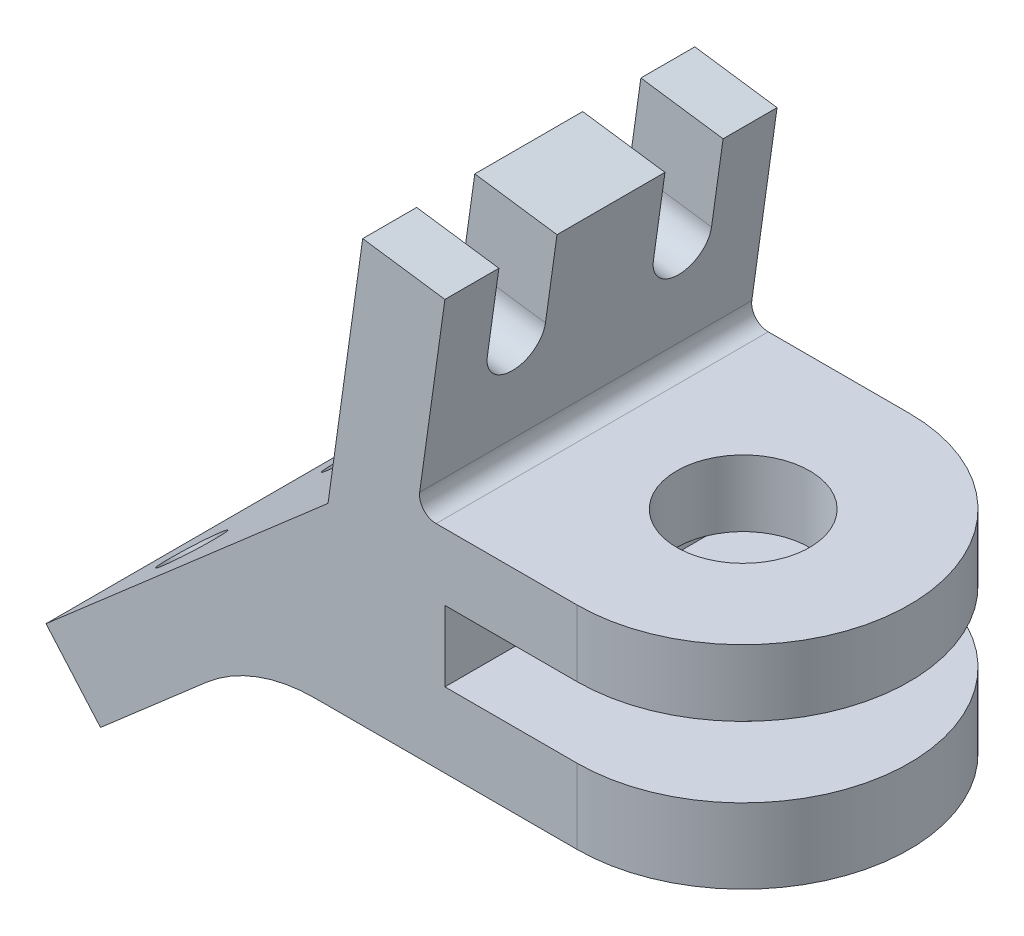
ISO-10303-21;
HEADER;
FILE_DESCRIPTION(('STEP AP214'),'2;1');
FILE_NAME('part.step','',(''),(''),'','','');
FILE_SCHEMA(('AUTOMOTIVE_DESIGN { 1 0 10303 214 1 1 1 1 }'));
ENDSEC;
DATA;
#1=APPLICATION_CONTEXT('core data for automotive mechanical design processes');
#2=APPLICATION_PROTOCOL_DEFINITION('international standard','automotive_design',2000,#1);
#3=PRODUCT_CONTEXT('',#1,'mechanical');
#4=PRODUCT('Part','Part','',(#3));
#5=PRODUCT_RELATED_PRODUCT_CATEGORY('part','',(#4));
#6=PRODUCT_DEFINITION_FORMATION('','',#4);
#7=PRODUCT_DEFINITION_CONTEXT('part definition',#1,'design');
#8=PRODUCT_DEFINITION('design','',#6,#7);
#9=PRODUCT_DEFINITION_SHAPE('','',#8);
#10=(LENGTH_UNIT() NAMED_UNIT(*) SI_UNIT(.MILLI.,.METRE.));
#11=(NAMED_UNIT(*) PLANE_ANGLE_UNIT() SI_UNIT($,.RADIAN.));
#12=(NAMED_UNIT(*) SI_UNIT($,.STERADIAN.) SOLID_ANGLE_UNIT());
#13=UNCERTAINTY_MEASURE_WITH_UNIT(LENGTH_MEASURE(1.E-05),#10,'distance_accuracy_value','');
#14=(GEOMETRIC_REPRESENTATION_CONTEXT(3) GLOBAL_UNCERTAINTY_ASSIGNED_CONTEXT((#13)) GLOBAL_UNIT_ASSIGNED_CONTEXT((#10,
#11,#12)) REPRESENTATION_CONTEXT('',''));
#15=CARTESIAN_POINT('',(0.,0.,0.));
#16=DIRECTION('',(0.,0.,1.));
#17=DIRECTION('',(1.,0.,0.));
#18=AXIS2_PLACEMENT_3D('',#15,#16,#17);
#19=CARTESIAN_POINT('',(0.,0.,4.));
#20=DIRECTION('',(-0.656059028990504,0.754709580222775,0.));
#21=DIRECTION('',(-0.754709580222775,-0.656059028990504,0.));
#22=AXIS2_PLACEMENT_3D('',#19,#20,#21);
#23=PLANE('',#22);
#24=CARTESIAN_POINT('',(-5.84731576057085,-5.08299404248799,-2.));
#25=DIRECTION('',(-0.656059028990504,0.754709580222775,0.));
#26=DIRECTION('',(-0.754709580222775,-0.656059028990504,0.));
#27=AXIS2_PLACEMENT_3D('',#24,#25,#26);
#28=CIRCLE('',#27,0.7);
#29=CARTESIAN_POINT('',(-6.37561246672679,-5.54223536278135,-2.));
#30=VERTEX_POINT('',#29);
#31=EDGE_CURVE('E244',#30,#30,#28,.T.);
#32=ORIENTED_EDGE('',*,*,#31,.T.);
#33=EDGE_LOOP('',(#32));
#34=FACE_BOUND('',#33,.T.);
#35=CARTESIAN_POINT('',(-5.84731576057085,-5.08299404248799,2.));
#36=DIRECTION('',(-0.656059028990504,0.754709580222775,0.));
#37=DIRECTION('',(-0.754709580222775,-0.656059028990504,0.));
#38=AXIS2_PLACEMENT_3D('',#35,#36,#37);
#39=CIRCLE('',#38,0.7);
#40=CARTESIAN_POINT('',(-6.37561246672679,-5.54223536278134,2.));
#41=VERTEX_POINT('',#40);
#42=EDGE_CURVE('E248',#41,#41,#39,.T.);
#43=ORIENTED_EDGE('',*,*,#42,.T.);
#44=EDGE_LOOP('',(#43));
#45=FACE_BOUND('',#44,.T.);
#46=DIRECTION('',(0.754709580222775,0.656059028990504,0.));
#47=VECTOR('',#46,1.);
#48=CARTESIAN_POINT('',(0.,0.,-4.));
#49=LINE('',#48,#47);
#50=CARTESIAN_POINT('',(-7.3567349210164,-6.395112100469,-4.));
#51=VERTEX_POINT('',#50);
#52=CARTESIAN_POINT('',(-4.80987630113007,-4.1811616791089,-4.));
#53=VERTEX_POINT('',#52);
#54=EDGE_CURVE('E325',#51,#53,#49,.T.);
#55=ORIENTED_EDGE('',*,*,#54,.T.);
#56=DIRECTION('',(0.,0.,-1.));
#57=VECTOR('',#56,1.);
#58=CARTESIAN_POINT('',(-4.80987630113007,-4.1811616791089,4.));
#59=LINE('',#58,#57);
#60=CARTESIAN_POINT('',(-4.80987630113007,-4.1811616791089,4.));
#61=VERTEX_POINT('',#60);
#62=EDGE_CURVE('E354',#53,#61,#59,.F.);
#63=ORIENTED_EDGE('',*,*,#62,.T.);
#64=DIRECTION('',(0.754709580222775,0.656059028990504,0.));
#65=VECTOR('',#64,1.);
#66=CARTESIAN_POINT('',(0.,0.,4.));
#67=LINE('',#66,#65);
#68=CARTESIAN_POINT('',(-7.3567349210164,-6.395112100469,4.));
#69=VERTEX_POINT('',#68);
#70=EDGE_CURVE('E306',#69,#61,#67,.T.);
#71=ORIENTED_EDGE('',*,*,#70,.F.);
#72=DIRECTION('',(0.,0.,-1.));
#73=VECTOR('',#72,1.);
#74=CARTESIAN_POINT('',(-7.3567349210164,-6.395112100469,4.));
#75=LINE('',#74,#73);
#76=EDGE_CURVE('E350',#69,#51,#75,.T.);
#77=ORIENTED_EDGE('',*,*,#76,.T.);
#78=EDGE_LOOP('',(#55,#63,#71,#77));
#79=FACE_BOUND('',#78,.T.);
#80=ADVANCED_FACE('F39',(#34,#45,#79),#23,.F.);
#81=CARTESIAN_POINT('',(0.939107986251134,6.68210053142036,4.));
#82=DIRECTION('',(-0.99026806874157,0.139173100960069,0.));
#83=DIRECTION('',(-0.139173100960069,-0.99026806874157,0.));
#84=AXIS2_PLACEMENT_3D('',#81,#82,#83);
#85=PLANE('',#84);
#86=DIRECTION('',(0.139173100960069,0.99026806874157,0.));
#87=VECTOR('',#86,1.);
#88=CARTESIAN_POINT('',(0.939107986251134,6.68210053142036,4.));
#89=LINE('',#88,#87);
#90=CARTESIAN_POINT('',(0.331067721326328,2.35566924038403,4.));
#91=VERTEX_POINT('',#90);
#92=CARTESIAN_POINT('',(0.939107986251134,6.68210053142036,4.));
#93=VERTEX_POINT('',#92);
#94=EDGE_CURVE('E313',#91,#93,#89,.T.);
#95=ORIENTED_EDGE('',*,*,#94,.F.);
#96=DIRECTION('',(0.,0.,-1.));
#97=VECTOR('',#96,1.);
#98=CARTESIAN_POINT('',(0.331067721326328,2.35566924038403,-4.));
#99=LINE('',#98,#97);
#100=CARTESIAN_POINT('',(0.331067721326328,2.35566924038403,-4.));
#101=VERTEX_POINT('',#100);
#102=EDGE_CURVE('E360',#91,#101,#99,.T.);
#103=ORIENTED_EDGE('',*,*,#102,.T.);
#104=DIRECTION('',(0.139173100960069,0.99026806874157,0.));
#105=VECTOR('',#104,1.);
#106=CARTESIAN_POINT('',(0.939107986251134,6.68210053142036,-4.));
#107=LINE('',#106,#105);
#108=CARTESIAN_POINT('',(0.939107986251134,6.68210053142036,-4.));
#109=VERTEX_POINT('',#108);
#110=EDGE_CURVE('E324',#101,#109,#107,.T.);
#111=ORIENTED_EDGE('',*,*,#110,.T.);
#112=DIRECTION('',(0.,0.,-1.));
#113=VECTOR('',#112,1.);
#114=CARTESIAN_POINT('',(0.939107986251134,6.68210053142036,4.));
#115=LINE('',#114,#113);
#116=CARTESIAN_POINT('',(0.939107986251136,6.68210053142036,-2.7));
#117=VERTEX_POINT('',#116);
#118=EDGE_CURVE('E342',#117,#109,#115,.T.);
#119=ORIENTED_EDGE('',*,*,#118,.F.);
#120=DIRECTION('',(-0.139173100960069,-0.99026806874157,0.));
#121=VECTOR('',#120,1.);
#122=CARTESIAN_POINT('',(0.939107986251134,6.68210053142036,-2.7));
#123=LINE('',#122,#121);
#124=CARTESIAN_POINT('',(0.660761784330996,4.70156439393722,-2.7));
#125=VERTEX_POINT('',#124);
#126=EDGE_CURVE('E298',#117,#125,#123,.T.);
#127=ORIENTED_EDGE('',*,*,#126,.T.);
#128=CARTESIAN_POINT('',(0.660761784330996,4.70156439393722,-2.));
#129=DIRECTION('',(-0.99026806874157,0.139173100960069,0.));
#130=DIRECTION('',(-0.139173100960069,-0.99026806874157,0.));
#131=AXIS2_PLACEMENT_3D('',#128,#129,#130);
#132=CIRCLE('',#131,0.7);
#133=CARTESIAN_POINT('',(0.660761784330996,4.70156439393722,-1.3));
#134=VERTEX_POINT('',#133);
#135=EDGE_CURVE('E301',#125,#134,#132,.T.);
#136=ORIENTED_EDGE('',*,*,#135,.T.);
#137=DIRECTION('',(0.139173100960069,0.99026806874157,0.));
#138=VECTOR('',#137,1.);
#139=CARTESIAN_POINT('',(0.939107986251134,6.68210053142036,-1.3));
#140=LINE('',#139,#138);
#141=CARTESIAN_POINT('',(0.939107986251136,6.68210053142036,-1.3));
#142=VERTEX_POINT('',#141);
#143=EDGE_CURVE('E293',#134,#142,#140,.T.);
#144=ORIENTED_EDGE('',*,*,#143,.T.);
#145=CARTESIAN_POINT('',(0.939107986251136,6.68210053142036,1.3));
#146=VERTEX_POINT('',#145);
#147=EDGE_CURVE('E346',#146,#142,#115,.T.);
#148=ORIENTED_EDGE('',*,*,#147,.F.);
#149=DIRECTION('',(-0.139173100960069,-0.99026806874157,0.));
#150=VECTOR('',#149,1.);
#151=CARTESIAN_POINT('',(0.939107986251134,6.68210053142036,1.3));
#152=LINE('',#151,#150);
#153=CARTESIAN_POINT('',(0.660761784330996,4.70156439393722,1.3));
#154=VERTEX_POINT('',#153);
#155=EDGE_CURVE('E288',#146,#154,#152,.T.);
#156=ORIENTED_EDGE('',*,*,#155,.T.);
#157=CARTESIAN_POINT('',(0.660761784330996,4.70156439393722,2.));
#158=DIRECTION('',(-0.99026806874157,0.139173100960069,0.));
#159=DIRECTION('',(-0.139173100960069,-0.99026806874157,0.));
#160=AXIS2_PLACEMENT_3D('',#157,#158,#159);
#161=CIRCLE('',#160,0.7);
#162=CARTESIAN_POINT('',(0.660761784330996,4.70156439393722,2.7));
#163=VERTEX_POINT('',#162);
#164=EDGE_CURVE('E295',#154,#163,#161,.T.);
#165=ORIENTED_EDGE('',*,*,#164,.T.);
#166=DIRECTION('',(0.139173100960069,0.99026806874157,0.));
#167=VECTOR('',#166,1.);
#168=CARTESIAN_POINT('',(0.939107986251134,6.68210053142036,2.7));
#169=LINE('',#168,#167);
#170=CARTESIAN_POINT('',(0.939107986251136,6.68210053142036,2.7));
#171=VERTEX_POINT('',#170);
#172=EDGE_CURVE('E262',#163,#171,#169,.T.);
#173=ORIENTED_EDGE('',*,*,#172,.T.);
#174=EDGE_CURVE('E343',#93,#171,#115,.T.);
#175=ORIENTED_EDGE('',*,*,#174,.F.);
#176=EDGE_LOOP('',(#95,#103,#111,#119,#127,#136,#144,#148,#156,#165,#173,#175));
#177=FACE_BOUND('',#176,.T.);
#178=ADVANCED_FACE('F368',(#177),#85,.F.);
#179=CARTESIAN_POINT('',(0.939107986251134,6.68210053142036,4.));
#180=DIRECTION('',(-0.13917310096007,-0.99026806874157,0.));
#181=DIRECTION('',(0.99026806874157,-0.13917310096007,0.));
#182=AXIS2_PLACEMENT_3D('',#179,#180,#181);
#183=PLANE('',#182);
#184=DIRECTION('',(0.,0.,-1.));
#185=VECTOR('',#184,1.);
#186=CARTESIAN_POINT('',(-1.04142815123201,6.9604467333405,4.));
#187=LINE('',#186,#185);
#188=CARTESIAN_POINT('',(-1.04142815123201,6.9604467333405,-2.7));
#189=VERTEX_POINT('',#188);
#190=CARTESIAN_POINT('',(-1.04142815123201,6.9604467333405,-4.));
#191=VERTEX_POINT('',#190);
#192=EDGE_CURVE('E338',#189,#191,#187,.T.);
#193=ORIENTED_EDGE('',*,*,#192,.F.);
#194=DIRECTION('',(-0.99026806874157,0.13917310096007,0.));
#195=VECTOR('',#194,1.);
#196=CARTESIAN_POINT('',(6.88071639870055,5.84706192565994,-2.7));
#197=LINE('',#196,#195);
#198=EDGE_CURVE('E264',#117,#189,#197,.T.);
#199=ORIENTED_EDGE('',*,*,#198,.F.);
#200=ORIENTED_EDGE('',*,*,#118,.T.);
#201=DIRECTION('',(-0.99026806874157,0.13917310096007,0.));
#202=VECTOR('',#201,1.);
#203=CARTESIAN_POINT('',(0.939107986251134,6.68210053142036,-4.));
#204=LINE('',#203,#202);
#205=EDGE_CURVE('E330',#109,#191,#204,.T.);
#206=ORIENTED_EDGE('',*,*,#205,.T.);
#207=EDGE_LOOP('',(#193,#199,#200,#206));
#208=FACE_BOUND('',#207,.T.);
#209=ADVANCED_FACE('F378',(#208),#183,.F.);
#210=ORIENTED_EDGE('',*,*,#147,.T.);
#211=DIRECTION('',(-0.99026806874157,0.13917310096007,0.));
#212=VECTOR('',#211,1.);
#213=CARTESIAN_POINT('',(6.88071639870055,5.84706192565994,-1.3));
#214=LINE('',#213,#212);
#215=CARTESIAN_POINT('',(-1.04142815123201,6.9604467333405,-1.3));
#216=VERTEX_POINT('',#215);
#217=EDGE_CURVE('E270',#142,#216,#214,.T.);
#218=ORIENTED_EDGE('',*,*,#217,.T.);
#219=CARTESIAN_POINT('',(-1.04142815123201,6.9604467333405,1.3));
#220=VERTEX_POINT('',#219);
#221=EDGE_CURVE('E344',#220,#216,#187,.T.);
#222=ORIENTED_EDGE('',*,*,#221,.F.);
#223=DIRECTION('',(-0.99026806874157,0.13917310096007,0.));
#224=VECTOR('',#223,1.);
#225=CARTESIAN_POINT('',(6.88071639870055,5.84706192565994,1.3));
#226=LINE('',#225,#224);
#227=EDGE_CURVE('E278',#146,#220,#226,.T.);
#228=ORIENTED_EDGE('',*,*,#227,.F.);
#229=EDGE_LOOP('',(#210,#218,#222,#228));
#230=FACE_BOUND('',#229,.T.);
#231=ADVANCED_FACE('F383',(#230),#183,.F.);
#232=CARTESIAN_POINT('',(-7.3567349210164,-6.395112100469,4.));
#233=DIRECTION('',(0.754709580222775,0.656059028990504,0.));
#234=DIRECTION('',(-0.656059028990504,0.754709580222775,0.));
#235=AXIS2_PLACEMENT_3D('',#232,#233,#234);
#236=PLANE('',#235);
#237=DIRECTION('',(0.656059028990504,-0.754709580222775,0.));
#238=VECTOR('',#237,1.);
#239=CARTESIAN_POINT('',(-7.3567349210164,-6.395112100469,-4.));
#240=LINE('',#239,#238);
#241=CARTESIAN_POINT('',(-8.6688529789974,-4.88569294002345,-4.));
#242=VERTEX_POINT('',#241);
#243=EDGE_CURVE('E303',#242,#51,#240,.T.);
#244=ORIENTED_EDGE('',*,*,#243,.T.);
#245=ORIENTED_EDGE('',*,*,#76,.F.);
#246=DIRECTION('',(0.656059028990504,-0.754709580222775,0.));
#247=VECTOR('',#246,1.);
#248=CARTESIAN_POINT('',(-7.3567349210164,-6.395112100469,4.));
#249=LINE('',#248,#247);
#250=CARTESIAN_POINT('',(-8.6688529789974,-4.88569294002345,4.));
#251=VERTEX_POINT('',#250);
#252=EDGE_CURVE('E305',#251,#69,#249,.T.);
#253=ORIENTED_EDGE('',*,*,#252,.F.);
#254=DIRECTION('',(0.,0.,-1.));
#255=VECTOR('',#254,1.);
#256=CARTESIAN_POINT('',(-8.6688529789974,-4.88569294002345,4.));
#257=LINE('',#256,#255);
#258=EDGE_CURVE('E317',#251,#242,#257,.T.);
#259=ORIENTED_EDGE('',*,*,#258,.T.);
#260=EDGE_LOOP('',(#244,#245,#253,#259));
#261=FACE_BOUND('',#260,.T.);
#262=ADVANCED_FACE('F409',(#261),#236,.F.);
#263=ORIENTED_EDGE('',*,*,#174,.T.);
#264=DIRECTION('',(-0.99026806874157,0.13917310096007,0.));
#265=VECTOR('',#264,1.);
#266=CARTESIAN_POINT('',(6.88071639870055,5.84706192565994,2.7));
#267=LINE('',#266,#265);
#268=CARTESIAN_POINT('',(-1.04142815123201,6.9604467333405,2.7));
#269=VERTEX_POINT('',#268);
#270=EDGE_CURVE('E285',#171,#269,#267,.T.);
#271=ORIENTED_EDGE('',*,*,#270,.T.);
#272=CARTESIAN_POINT('',(-1.04142815123201,6.9604467333405,4.));
#273=VERTEX_POINT('',#272);
#274=EDGE_CURVE('E339',#273,#269,#187,.T.);
#275=ORIENTED_EDGE('',*,*,#274,.F.);
#276=DIRECTION('',(-0.99026806874157,0.13917310096007,0.));
#277=VECTOR('',#276,1.);
#278=CARTESIAN_POINT('',(0.939107986251134,6.68210053142036,4.));
#279=LINE('',#278,#277);
#280=EDGE_CURVE('E311',#93,#273,#279,.T.);
#281=ORIENTED_EDGE('',*,*,#280,.F.);
#282=EDGE_LOOP('',(#263,#271,#275,#281));
#283=FACE_BOUND('',#282,.T.);
#284=ADVANCED_FACE('F418',(#283),#183,.F.);
#285=CARTESIAN_POINT('',(-1.87646675699242,1.01883832089108,4.));
#286=DIRECTION('',(0.99026806874157,-0.13917310096007,0.));
#287=DIRECTION('',(0.13917310096007,0.99026806874157,0.));
#288=AXIS2_PLACEMENT_3D('',#285,#286,#287);
#289=PLANE('',#288);
#290=CARTESIAN_POINT('',(-1.31977435315215,4.97991059585736,-2.));
#291=DIRECTION('',(-0.99026806874157,0.13917310096007,0.));
#292=DIRECTION('',(-0.13917310096007,-0.99026806874157,0.));
#293=AXIS2_PLACEMENT_3D('',#290,#291,#292);
#294=CIRCLE('',#293,0.7);
#295=CARTESIAN_POINT('',(-1.31977435315215,4.97991059585736,-2.7));
#296=VERTEX_POINT('',#295);
#297=CARTESIAN_POINT('',(-1.31977435315215,4.97991059585736,-1.3));
#298=VERTEX_POINT('',#297);
#299=EDGE_CURVE('E251',#296,#298,#294,.T.);
#300=ORIENTED_EDGE('',*,*,#299,.F.);
#301=DIRECTION('',(-0.13917310096007,-0.99026806874157,0.));
#302=VECTOR('',#301,1.);
#303=CARTESIAN_POINT('',(-1.31977435315215,4.97991059585736,-2.7));
#304=LINE('',#303,#302);
#305=EDGE_CURVE('E256',#189,#296,#304,.T.);
#306=ORIENTED_EDGE('',*,*,#305,.F.);
#307=ORIENTED_EDGE('',*,*,#192,.T.);
#308=DIRECTION('',(-0.13917310096007,-0.99026806874157,0.));
#309=VECTOR('',#308,1.);
#310=CARTESIAN_POINT('',(-1.87646675699242,1.01883832089108,-4.));
#311=LINE('',#310,#309);
#312=CARTESIAN_POINT('',(-1.87646675699242,1.01883832089108,-4.));
#313=VERTEX_POINT('',#312);
#314=EDGE_CURVE('E329',#191,#313,#311,.T.);
#315=ORIENTED_EDGE('',*,*,#314,.T.);
#316=DIRECTION('',(0.,0.,-1.));
#317=VECTOR('',#316,1.);
#318=CARTESIAN_POINT('',(-1.87646675699242,1.01883832089108,4.));
#319=LINE('',#318,#317);
#320=CARTESIAN_POINT('',(-1.87646675699242,1.01883832089108,4.));
#321=VERTEX_POINT('',#320);
#322=EDGE_CURVE('E333',#321,#313,#319,.T.);
#323=ORIENTED_EDGE('',*,*,#322,.F.);
#324=DIRECTION('',(-0.13917310096007,-0.99026806874157,0.));
#325=VECTOR('',#324,1.);
#326=CARTESIAN_POINT('',(-1.87646675699242,1.01883832089108,4.));
#327=LINE('',#326,#325);
#328=EDGE_CURVE('E312',#273,#321,#327,.T.);
#329=ORIENTED_EDGE('',*,*,#328,.F.);
#330=ORIENTED_EDGE('',*,*,#274,.T.);
#331=DIRECTION('',(0.13917310096007,0.99026806874157,0.));
#332=VECTOR('',#331,1.);
#333=CARTESIAN_POINT('',(-1.31977435315215,4.97991059585736,2.7));
#334=LINE('',#333,#332);
#335=CARTESIAN_POINT('',(-1.31977435315215,4.97991059585736,2.7));
#336=VERTEX_POINT('',#335);
#337=EDGE_CURVE('E272',#336,#269,#334,.T.);
#338=ORIENTED_EDGE('',*,*,#337,.F.);
#339=CARTESIAN_POINT('',(-1.31977435315215,4.97991059585736,2.));
#340=DIRECTION('',(-0.99026806874157,0.13917310096007,0.));
#341=DIRECTION('',(0.13917310096007,0.99026806874157,0.));
#342=AXIS2_PLACEMENT_3D('',#339,#340,#341);
#343=CIRCLE('',#342,0.7);
#344=CARTESIAN_POINT('',(-1.31977435315215,4.97991059585736,1.3));
#345=VERTEX_POINT('',#344);
#346=EDGE_CURVE('E252',#345,#336,#343,.T.);
#347=ORIENTED_EDGE('',*,*,#346,.F.);
#348=DIRECTION('',(-0.13917310096007,-0.99026806874157,0.));
#349=VECTOR('',#348,1.);
#350=CARTESIAN_POINT('',(-1.04142815123201,6.9604467333405,1.3));
#351=LINE('',#350,#349);
#352=EDGE_CURVE('E274',#220,#345,#351,.T.);
#353=ORIENTED_EDGE('',*,*,#352,.F.);
#354=ORIENTED_EDGE('',*,*,#221,.T.);
#355=DIRECTION('',(0.13917310096007,0.99026806874157,0.));
#356=VECTOR('',#355,1.);
#357=CARTESIAN_POINT('',(-1.04142815123201,6.9604467333405,-1.3));
#358=LINE('',#357,#356);
#359=EDGE_CURVE('E254',#298,#216,#358,.T.);
#360=ORIENTED_EDGE('',*,*,#359,.F.);
#361=EDGE_LOOP('',(#300,#306,#307,#315,#323,#329,#330,#338,#347,#353,#354,#360));
#362=FACE_BOUND('',#361,.T.);
#363=ADVANCED_FACE('F397',(#362),#289,.F.);
#364=CARTESIAN_POINT('',(-8.6688529789974,-4.88569294002345,4.));
#365=DIRECTION('',(0.656059028990503,-0.754709580222775,0.));
#366=DIRECTION('',(0.754709580222775,0.656059028990503,0.));
#367=AXIS2_PLACEMENT_3D('',#364,#365,#366);
#368=PLANE('',#367);
#369=CARTESIAN_POINT('',(-7.15943381855185,-3.57357488204244,2.));
#370=DIRECTION('',(-0.656059028990504,0.754709580222775,0.));
#371=DIRECTION('',(-0.754709580222775,-0.656059028990504,0.));
#372=AXIS2_PLACEMENT_3D('',#369,#370,#371);
#373=CIRCLE('',#372,0.7);
#374=CARTESIAN_POINT('',(-7.6877305247078,-4.03281620233579,2.));
#375=VERTEX_POINT('',#374);
#376=EDGE_CURVE('E242',#375,#375,#373,.T.);
#377=ORIENTED_EDGE('',*,*,#376,.F.);
#378=EDGE_LOOP('',(#377));
#379=FACE_BOUND('',#378,.T.);
#380=CARTESIAN_POINT('',(-7.15943381855185,-3.57357488204244,-2.));
#381=DIRECTION('',(-0.656059028990504,0.754709580222775,0.));
#382=DIRECTION('',(-0.754709580222775,-0.656059028990504,0.));
#383=AXIS2_PLACEMENT_3D('',#380,#381,#382);
#384=CIRCLE('',#383,0.7);
#385=CARTESIAN_POINT('',(-7.6877305247078,-4.03281620233579,-2.));
#386=VERTEX_POINT('',#385);
#387=EDGE_CURVE('E238',#386,#386,#384,.T.);
#388=ORIENTED_EDGE('',*,*,#387,.F.);
#389=EDGE_LOOP('',(#388));
#390=FACE_BOUND('',#389,.T.);
#391=DIRECTION('',(-0.754709580222775,-0.656059028990503,0.));
#392=VECTOR('',#391,1.);
#393=CARTESIAN_POINT('',(-8.6688529789974,-4.88569294002345,-4.));
#394=LINE('',#393,#392);
#395=EDGE_CURVE('E310',#313,#242,#394,.T.);
#396=ORIENTED_EDGE('',*,*,#395,.T.);
#397=ORIENTED_EDGE('',*,*,#258,.F.);
#398=DIRECTION('',(-0.754709580222775,-0.656059028990503,0.));
#399=VECTOR('',#398,1.);
#400=CARTESIAN_POINT('',(-8.6688529789974,-4.88569294002345,4.));
#401=LINE('',#400,#399);
#402=EDGE_CURVE('E320',#321,#251,#401,.T.);
#403=ORIENTED_EDGE('',*,*,#402,.F.);
#404=ORIENTED_EDGE('',*,*,#322,.T.);
#405=EDGE_LOOP('',(#396,#397,#403,#404));
#406=FACE_BOUND('',#405,.T.);
#407=ADVANCED_FACE('F404',(#379,#390,#406),#368,.F.);
#408=CARTESIAN_POINT('',(0.,0.,4.));
#409=DIRECTION('',(0.,0.,-1.));
#410=DIRECTION('',(-1.,0.,0.));
#411=AXIS2_PLACEMENT_3D('',#408,#409,#410);
#412=PLANE('',#411);
#413=ORIENTED_EDGE('',*,*,#70,.T.);
#414=CARTESIAN_POINT('',(-2.18564018516806,-7.2,4.));
#415=DIRECTION('',(0.,0.,-1.));
#416=DIRECTION('',(-1.,0.,0.));
#417=AXIS2_PLACEMENT_3D('',#414,#415,#416);
#418=CIRCLE('',#417,4.);
#419=CARTESIAN_POINT('',(-2.18564018516806,-3.2,4.));
#420=VERTEX_POINT('',#419);
#421=EDGE_CURVE('E359',#61,#420,#418,.T.);
#422=ORIENTED_EDGE('',*,*,#421,.T.);
#423=DIRECTION('',(1.,0.,0.));
#424=VECTOR('',#423,1.);
#425=CARTESIAN_POINT('',(-3.68117890310727,-3.2,4.));
#426=LINE('',#425,#424);
#427=CARTESIAN_POINT('',(4.12353324300758,-3.2,4.));
#428=VERTEX_POINT('',#427);
#429=EDGE_CURVE('E237',#420,#428,#426,.T.);
#430=ORIENTED_EDGE('',*,*,#429,.T.);
#431=DIRECTION('',(0.,1.,0.));
#432=VECTOR('',#431,1.);
#433=CARTESIAN_POINT('',(4.12353324300758,-3.2,4.));
#434=LINE('',#433,#432);
#435=CARTESIAN_POINT('',(4.12353324300758,-1.4,4.));
#436=VERTEX_POINT('',#435);
#437=EDGE_CURVE('E461',#428,#436,#434,.T.);
#438=ORIENTED_EDGE('',*,*,#437,.T.);
#439=DIRECTION('',(-1.,0.,0.));
#440=VECTOR('',#439,1.);
#441=CARTESIAN_POINT('',(4.12353324300758,-1.4,4.));
#442=LINE('',#441,#440);
#443=CARTESIAN_POINT('',(0.939107986251134,-1.4,4.));
#444=VERTEX_POINT('',#443);
#445=EDGE_CURVE('E467',#436,#444,#442,.T.);
#446=ORIENTED_EDGE('',*,*,#445,.T.);
#447=DIRECTION('',(0.,1.,0.));
#448=VECTOR('',#447,1.);
#449=CARTESIAN_POINT('',(0.939107986251134,-1.4,4.));
#450=LINE('',#449,#448);
#451=CARTESIAN_POINT('',(0.939107986251134,0.3,4.));
#452=VERTEX_POINT('',#451);
#453=EDGE_CURVE('E475',#444,#452,#450,.T.);
#454=ORIENTED_EDGE('',*,*,#453,.T.);
#455=DIRECTION('',(1.,0.,0.));
#456=VECTOR('',#455,1.);
#457=CARTESIAN_POINT('',(0.939107986251134,0.3,4.));
#458=LINE('',#457,#456);
#459=CARTESIAN_POINT('',(4.12353324300758,0.3,4.));
#460=VERTEX_POINT('',#459);
#461=EDGE_CURVE('E209',#452,#460,#458,.T.);
#462=ORIENTED_EDGE('',*,*,#461,.T.);
#463=DIRECTION('',(0.,1.,0.));
#464=VECTOR('',#463,1.);
#465=CARTESIAN_POINT('',(4.12353324300758,0.3,4.));
#466=LINE('',#465,#464);
#467=CARTESIAN_POINT('',(4.12353324300758,1.9,4.));
#468=VERTEX_POINT('',#467);
#469=EDGE_CURVE('E197',#460,#468,#466,.T.);
#470=ORIENTED_EDGE('',*,*,#469,.T.);
#471=DIRECTION('',(-1.,0.,0.));
#472=VECTOR('',#471,1.);
#473=CARTESIAN_POINT('',(4.12353324300758,1.9,4.));
#474=LINE('',#473,#472);
#475=CARTESIAN_POINT('',(0.727174948822957,1.9,4.));
#476=VERTEX_POINT('',#475);
#477=EDGE_CURVE('E210',#468,#476,#474,.T.);
#478=ORIENTED_EDGE('',*,*,#477,.T.);
#479=CARTESIAN_POINT('',(0.727174948822956,2.3,4.));
#480=DIRECTION('',(0.,0.,-1.));
#481=DIRECTION('',(-1.,0.,0.));
#482=AXIS2_PLACEMENT_3D('',#479,#480,#481);
#483=CIRCLE('',#482,0.4);
#484=EDGE_CURVE('E11',#476,#91,#483,.T.);
#485=ORIENTED_EDGE('',*,*,#484,.T.);
#486=ORIENTED_EDGE('',*,*,#94,.T.);
#487=ORIENTED_EDGE('',*,*,#280,.T.);
#488=ORIENTED_EDGE('',*,*,#328,.T.);
#489=ORIENTED_EDGE('',*,*,#402,.T.);
#490=ORIENTED_EDGE('',*,*,#252,.T.);
#491=EDGE_LOOP('',(#413,#422,#430,#438,#446,#454,#462,#470,#478,#485,#486,#487,#488,#489,#490));
#492=FACE_BOUND('',#491,.T.);
#493=ADVANCED_FACE('F206',(#492),#412,.F.);
#494=CARTESIAN_POINT('',(0.,0.,-4.));
#495=DIRECTION('',(0.,0.,-1.));
#496=DIRECTION('',(-1.,0.,0.));
#497=AXIS2_PLACEMENT_3D('',#494,#495,#496);
#498=PLANE('',#497);
#499=DIRECTION('',(1.,0.,0.));
#500=VECTOR('',#499,1.);
#501=CARTESIAN_POINT('',(-3.68117890310727,-3.2,-4.));
#502=LINE('',#501,#500);
#503=CARTESIAN_POINT('',(-2.18564018516806,-3.2,-4.));
#504=VERTEX_POINT('',#503);
#505=CARTESIAN_POINT('',(4.12353324300758,-3.2,-4.));
#506=VERTEX_POINT('',#505);
#507=EDGE_CURVE('E219',#504,#506,#502,.T.);
#508=ORIENTED_EDGE('',*,*,#507,.F.);
#509=CARTESIAN_POINT('',(-2.18564018516806,-7.2,-4.));
#510=DIRECTION('',(0.,0.,-1.));
#511=DIRECTION('',(-1.,0.,0.));
#512=AXIS2_PLACEMENT_3D('',#509,#510,#511);
#513=CIRCLE('',#512,4.);
#514=EDGE_CURVE('E356',#504,#53,#513,.F.);
#515=ORIENTED_EDGE('',*,*,#514,.T.);
#516=ORIENTED_EDGE('',*,*,#54,.F.);
#517=ORIENTED_EDGE('',*,*,#243,.F.);
#518=ORIENTED_EDGE('',*,*,#395,.F.);
#519=ORIENTED_EDGE('',*,*,#314,.F.);
#520=ORIENTED_EDGE('',*,*,#205,.F.);
#521=ORIENTED_EDGE('',*,*,#110,.F.);
#522=CARTESIAN_POINT('',(0.727174948822956,2.3,-4.));
#523=DIRECTION('',(0.,0.,-1.));
#524=DIRECTION('',(-1.,0.,0.));
#525=AXIS2_PLACEMENT_3D('',#522,#523,#524);
#526=CIRCLE('',#525,0.4);
#527=CARTESIAN_POINT('',(0.727174948822957,1.9,-4.));
#528=VERTEX_POINT('',#527);
#529=EDGE_CURVE('E50',#101,#528,#526,.F.);
#530=ORIENTED_EDGE('',*,*,#529,.T.);
#531=DIRECTION('',(-1.,0.,0.));
#532=VECTOR('',#531,1.);
#533=CARTESIAN_POINT('',(4.12353324300758,1.9,-4.));
#534=LINE('',#533,#532);
#535=CARTESIAN_POINT('',(4.12353324300758,1.9,-4.));
#536=VERTEX_POINT('',#535);
#537=EDGE_CURVE('E235',#536,#528,#534,.T.);
#538=ORIENTED_EDGE('',*,*,#537,.F.);
#539=DIRECTION('',(0.,1.,0.));
#540=VECTOR('',#539,1.);
#541=CARTESIAN_POINT('',(4.12353324300758,0.3,-4.));
#542=LINE('',#541,#540);
#543=CARTESIAN_POINT('',(4.12353324300758,0.3,-4.));
#544=VERTEX_POINT('',#543);
#545=EDGE_CURVE('E199',#544,#536,#542,.T.);
#546=ORIENTED_EDGE('',*,*,#545,.F.);
#547=DIRECTION('',(1.,0.,0.));
#548=VECTOR('',#547,1.);
#549=CARTESIAN_POINT('',(0.939107986251134,0.3,-4.));
#550=LINE('',#549,#548);
#551=CARTESIAN_POINT('',(0.939107986251134,0.3,-4.));
#552=VERTEX_POINT('',#551);
#553=EDGE_CURVE('E231',#552,#544,#550,.T.);
#554=ORIENTED_EDGE('',*,*,#553,.F.);
#555=DIRECTION('',(0.,1.,0.));
#556=VECTOR('',#555,1.);
#557=CARTESIAN_POINT('',(0.939107986251134,-1.4,-4.));
#558=LINE('',#557,#556);
#559=CARTESIAN_POINT('',(0.939107986251134,-1.4,-4.));
#560=VERTEX_POINT('',#559);
#561=EDGE_CURVE('E229',#560,#552,#558,.T.);
#562=ORIENTED_EDGE('',*,*,#561,.F.);
#563=DIRECTION('',(-1.,0.,0.));
#564=VECTOR('',#563,1.);
#565=CARTESIAN_POINT('',(4.12353324300758,-1.4,-4.));
#566=LINE('',#565,#564);
#567=CARTESIAN_POINT('',(4.12353324300758,-1.4,-4.));
#568=VERTEX_POINT('',#567);
#569=EDGE_CURVE('E230',#568,#560,#566,.T.);
#570=ORIENTED_EDGE('',*,*,#569,.F.);
#571=DIRECTION('',(0.,1.,0.));
#572=VECTOR('',#571,1.);
#573=CARTESIAN_POINT('',(4.12353324300758,-3.2,-4.));
#574=LINE('',#573,#572);
#575=EDGE_CURVE('E224',#506,#568,#574,.T.);
#576=ORIENTED_EDGE('',*,*,#575,.F.);
#577=EDGE_LOOP('',(#508,#515,#516,#517,#518,#519,#520,#521,#530,#538,#546,#554,#562,#570,#576));
#578=FACE_BOUND('',#577,.T.);
#579=ADVANCED_FACE('F373',(#578),#498,.T.);
#580=CARTESIAN_POINT('',(6.60237019678041,3.8665257881768,2.));
#581=DIRECTION('',(-0.99026806874157,0.13917310096007,0.));
#582=DIRECTION('',(-0.13917310096007,-0.99026806874157,0.));
#583=AXIS2_PLACEMENT_3D('',#580,#581,#582);
#584=CYLINDRICAL_SURFACE('',#583,0.7);
#585=DIRECTION('',(-0.99026806874157,0.13917310096007,0.));
#586=VECTOR('',#585,1.);
#587=CARTESIAN_POINT('',(6.60237019678041,3.8665257881768,1.3));
#588=LINE('',#587,#586);
#589=EDGE_CURVE('E258',#154,#345,#588,.T.);
#590=ORIENTED_EDGE('',*,*,#589,.T.);
#591=ORIENTED_EDGE('',*,*,#346,.T.);
#592=DIRECTION('',(-0.99026806874157,0.13917310096007,0.));
#593=VECTOR('',#592,1.);
#594=CARTESIAN_POINT('',(6.60237019678041,3.8665257881768,2.7));
#595=LINE('',#594,#593);
#596=EDGE_CURVE('E279',#163,#336,#595,.T.);
#597=ORIENTED_EDGE('',*,*,#596,.F.);
#598=ORIENTED_EDGE('',*,*,#164,.F.);
#599=EDGE_LOOP('',(#590,#591,#597,#598));
#600=FACE_BOUND('',#599,.T.);
#601=ADVANCED_FACE('F425',(#600),#584,.F.);
#602=CARTESIAN_POINT('',(6.88071639870055,5.84706192565994,1.3));
#603=DIRECTION('',(0.,0.,-1.));
#604=DIRECTION('',(0.,1.,0.));
#605=AXIS2_PLACEMENT_3D('',#602,#603,#604);
#606=PLANE('',#605);
#607=ORIENTED_EDGE('',*,*,#227,.T.);
#608=ORIENTED_EDGE('',*,*,#352,.T.);
#609=ORIENTED_EDGE('',*,*,#589,.F.);
#610=ORIENTED_EDGE('',*,*,#155,.F.);
#611=EDGE_LOOP('',(#607,#608,#609,#610));
#612=FACE_BOUND('',#611,.T.);
#613=ADVANCED_FACE('F424',(#612),#606,.F.);
#614=CARTESIAN_POINT('',(6.60237019678041,3.8665257881768,2.7));
#615=DIRECTION('',(0.,0.,1.));
#616=DIRECTION('',(0.,-1.,0.));
#617=AXIS2_PLACEMENT_3D('',#614,#615,#616);
#618=PLANE('',#617);
#619=ORIENTED_EDGE('',*,*,#596,.T.);
#620=ORIENTED_EDGE('',*,*,#337,.T.);
#621=ORIENTED_EDGE('',*,*,#270,.F.);
#622=ORIENTED_EDGE('',*,*,#172,.F.);
#623=EDGE_LOOP('',(#619,#620,#621,#622));
#624=FACE_BOUND('',#623,.T.);
#625=ADVANCED_FACE('F416',(#624),#618,.F.);
#626=CARTESIAN_POINT('',(6.60237019678041,3.8665257881768,-2.));
#627=DIRECTION('',(-0.99026806874157,0.13917310096007,0.));
#628=DIRECTION('',(-0.13917310096007,-0.99026806874157,0.));
#629=AXIS2_PLACEMENT_3D('',#626,#627,#628);
#630=CYLINDRICAL_SURFACE('',#629,0.7);
#631=DIRECTION('',(-0.99026806874157,0.13917310096007,0.));
#632=VECTOR('',#631,1.);
#633=CARTESIAN_POINT('',(6.60237019678041,3.8665257881768,-2.7));
#634=LINE('',#633,#632);
#635=EDGE_CURVE('E265',#125,#296,#634,.T.);
#636=ORIENTED_EDGE('',*,*,#635,.T.);
#637=ORIENTED_EDGE('',*,*,#299,.T.);
#638=DIRECTION('',(-0.99026806874157,0.13917310096007,0.));
#639=VECTOR('',#638,1.);
#640=CARTESIAN_POINT('',(6.60237019678041,3.8665257881768,-1.3));
#641=LINE('',#640,#639);
#642=EDGE_CURVE('E261',#134,#298,#641,.T.);
#643=ORIENTED_EDGE('',*,*,#642,.F.);
#644=ORIENTED_EDGE('',*,*,#135,.F.);
#645=EDGE_LOOP('',(#636,#637,#643,#644));
#646=FACE_BOUND('',#645,.T.);
#647=ADVANCED_FACE('F395',(#646),#630,.F.);
#648=CARTESIAN_POINT('',(6.60237019678041,3.8665257881768,-2.7));
#649=DIRECTION('',(0.,0.,-1.));
#650=DIRECTION('',(0.,1.,0.));
#651=AXIS2_PLACEMENT_3D('',#648,#649,#650);
#652=PLANE('',#651);
#653=ORIENTED_EDGE('',*,*,#198,.T.);
#654=ORIENTED_EDGE('',*,*,#305,.T.);
#655=ORIENTED_EDGE('',*,*,#635,.F.);
#656=ORIENTED_EDGE('',*,*,#126,.F.);
#657=EDGE_LOOP('',(#653,#654,#655,#656));
#658=FACE_BOUND('',#657,.T.);
#659=ADVANCED_FACE('F527',(#658),#652,.F.);
#660=CARTESIAN_POINT('',(6.88071639870055,5.84706192565994,-1.3));
#661=DIRECTION('',(0.,0.,1.));
#662=DIRECTION('',(0.,-1.,0.));
#663=AXIS2_PLACEMENT_3D('',#660,#661,#662);
#664=PLANE('',#663);
#665=ORIENTED_EDGE('',*,*,#642,.T.);
#666=ORIENTED_EDGE('',*,*,#359,.T.);
#667=ORIENTED_EDGE('',*,*,#217,.F.);
#668=ORIENTED_EDGE('',*,*,#143,.F.);
#669=EDGE_LOOP('',(#665,#666,#667,#668));
#670=FACE_BOUND('',#669,.T.);
#671=ADVANCED_FACE('F386',(#670),#664,.F.);
#672=CARTESIAN_POINT('',(-2.27667339817812,-9.19054820966963,-2.));
#673=DIRECTION('',(-0.656059028990503,0.754709580222775,0.));
#674=DIRECTION('',(-0.754709580222775,-0.656059028990503,0.));
#675=AXIS2_PLACEMENT_3D('',#672,#673,#674);
#676=CYLINDRICAL_SURFACE('',#675,0.7);
#677=ORIENTED_EDGE('',*,*,#387,.T.);
#678=EDGE_LOOP('',(#677));
#679=FACE_BOUND('',#678,.T.);
#680=ORIENTED_EDGE('',*,*,#31,.F.);
#681=EDGE_LOOP('',(#680));
#682=FACE_BOUND('',#681,.T.);
#683=ADVANCED_FACE('F522',(#679,#682),#676,.F.);
#684=CARTESIAN_POINT('',(-2.27667339817812,-9.19054820966962,2.));
#685=DIRECTION('',(-0.656059028990503,0.754709580222775,0.));
#686=DIRECTION('',(-0.754709580222775,-0.656059028990503,0.));
#687=AXIS2_PLACEMENT_3D('',#684,#685,#686);
#688=CYLINDRICAL_SURFACE('',#687,0.7);
#689=ORIENTED_EDGE('',*,*,#376,.T.);
#690=EDGE_LOOP('',(#689));
#691=FACE_BOUND('',#690,.T.);
#692=ORIENTED_EDGE('',*,*,#42,.F.);
#693=EDGE_LOOP('',(#692));
#694=FACE_BOUND('',#693,.T.);
#695=ADVANCED_FACE('F518',(#691,#694),#688,.F.);
#696=CARTESIAN_POINT('',(-3.68117890310727,-3.2,4.));
#697=DIRECTION('',(0.,1.,0.));
#698=DIRECTION('',(-1.,0.,0.));
#699=AXIS2_PLACEMENT_3D('',#696,#697,#698);
#700=PLANE('',#699);
#701=CARTESIAN_POINT('',(4.12353324300758,-3.2,0.));
#702=DIRECTION('',(0.,1.,0.));
#703=DIRECTION('',(-1.,0.,0.));
#704=AXIS2_PLACEMENT_3D('',#701,#702,#703);
#705=CIRCLE('',#704,1.6);
#706=CARTESIAN_POINT('',(2.52353324300758,-3.2,0.));
#707=VERTEX_POINT('',#706);
#708=EDGE_CURVE('E205',#707,#707,#705,.T.);
#709=ORIENTED_EDGE('',*,*,#708,.T.);
#710=EDGE_LOOP('',(#709));
#711=FACE_BOUND('',#710,.T.);
#712=ORIENTED_EDGE('',*,*,#429,.F.);
#713=DIRECTION('',(0.,0.,-1.));
#714=VECTOR('',#713,1.);
#715=CARTESIAN_POINT('',(-2.18564018516806,-3.2,-4.));
#716=LINE('',#715,#714);
#717=EDGE_CURVE('E352',#420,#504,#716,.T.);
#718=ORIENTED_EDGE('',*,*,#717,.T.);
#719=ORIENTED_EDGE('',*,*,#507,.T.);
#720=CARTESIAN_POINT('',(4.12353324300758,-3.2,0.));
#721=DIRECTION('',(0.,1.,0.));
#722=DIRECTION('',(-1.,0.,0.));
#723=AXIS2_PLACEMENT_3D('',#720,#721,#722);
#724=CIRCLE('',#723,4.);
#725=EDGE_CURVE('E221',#506,#428,#724,.F.);
#726=ORIENTED_EDGE('',*,*,#725,.T.);
#727=EDGE_LOOP('',(#712,#718,#719,#726));
#728=FACE_BOUND('',#727,.T.);
#729=ADVANCED_FACE('F463',(#711,#728),#700,.F.);
#730=CARTESIAN_POINT('',(4.12353324300758,-1.4,4.));
#731=DIRECTION('',(0.,-1.,0.));
#732=DIRECTION('',(1.,0.,0.));
#733=AXIS2_PLACEMENT_3D('',#730,#731,#732);
#734=PLANE('',#733);
#735=CARTESIAN_POINT('',(4.12353324300758,-1.4,0.));
#736=DIRECTION('',(0.,-1.,0.));
#737=DIRECTION('',(1.,0.,0.));
#738=AXIS2_PLACEMENT_3D('',#735,#736,#737);
#739=CIRCLE('',#738,1.6);
#740=CARTESIAN_POINT('',(5.72353324300758,-1.4,0.));
#741=VERTEX_POINT('',#740);
#742=EDGE_CURVE('E488',#741,#741,#739,.T.);
#743=ORIENTED_EDGE('',*,*,#742,.T.);
#744=EDGE_LOOP('',(#743));
#745=FACE_BOUND('',#744,.T.);
#746=ORIENTED_EDGE('',*,*,#569,.T.);
#747=DIRECTION('',(0.,0.,-1.));
#748=VECTOR('',#747,1.);
#749=CARTESIAN_POINT('',(0.939107986251134,-1.4,4.));
#750=LINE('',#749,#748);
#751=EDGE_CURVE('E216',#444,#560,#750,.T.);
#752=ORIENTED_EDGE('',*,*,#751,.F.);
#753=ORIENTED_EDGE('',*,*,#445,.F.);
#754=CARTESIAN_POINT('',(4.12353324300758,-1.4,0.));
#755=DIRECTION('',(0.,1.,0.));
#756=DIRECTION('',(1.,0.,0.));
#757=AXIS2_PLACEMENT_3D('',#754,#755,#756);
#758=CIRCLE('',#757,4.);
#759=EDGE_CURVE('E470',#436,#568,#758,.T.);
#760=ORIENTED_EDGE('',*,*,#759,.T.);
#761=EDGE_LOOP('',(#746,#752,#753,#760));
#762=FACE_BOUND('',#761,.T.);
#763=ADVANCED_FACE('F510',(#745,#762),#734,.F.);
#764=CARTESIAN_POINT('',(0.939107986251134,-1.4,4.));
#765=DIRECTION('',(-1.,0.,0.));
#766=DIRECTION('',(0.,0.,1.));
#767=AXIS2_PLACEMENT_3D('',#764,#765,#766);
#768=PLANE('',#767);
#769=ORIENTED_EDGE('',*,*,#561,.T.);
#770=DIRECTION('',(0.,0.,-1.));
#771=VECTOR('',#770,1.);
#772=CARTESIAN_POINT('',(0.939107986251134,0.3,4.));
#773=LINE('',#772,#771);
#774=EDGE_CURVE('E213',#452,#552,#773,.T.);
#775=ORIENTED_EDGE('',*,*,#774,.F.);
#776=ORIENTED_EDGE('',*,*,#453,.F.);
#777=ORIENTED_EDGE('',*,*,#751,.T.);
#778=EDGE_LOOP('',(#769,#775,#776,#777));
#779=FACE_BOUND('',#778,.T.);
#780=ADVANCED_FACE('F477',(#779),#768,.F.);
#781=CARTESIAN_POINT('',(0.939107986251134,0.3,4.));
#782=DIRECTION('',(0.,1.,0.));
#783=DIRECTION('',(0.,0.,1.));
#784=AXIS2_PLACEMENT_3D('',#781,#782,#783);
#785=PLANE('',#784);
#786=CARTESIAN_POINT('',(4.12353324300758,0.3,0.));
#787=DIRECTION('',(0.,1.,0.));
#788=DIRECTION('',(0.,0.,1.));
#789=AXIS2_PLACEMENT_3D('',#786,#787,#788);
#790=CIRCLE('',#789,1.6);
#791=CARTESIAN_POINT('',(4.12353324300758,0.3,1.6));
#792=VERTEX_POINT('',#791);
#793=EDGE_CURVE('E491',#792,#792,#790,.T.);
#794=ORIENTED_EDGE('',*,*,#793,.T.);
#795=EDGE_LOOP('',(#794));
#796=FACE_BOUND('',#795,.T.);
#797=ORIENTED_EDGE('',*,*,#553,.T.);
#798=CARTESIAN_POINT('',(4.12353324300758,0.3,0.));
#799=DIRECTION('',(0.,1.,0.));
#800=DIRECTION('',(0.,0.,1.));
#801=AXIS2_PLACEMENT_3D('',#798,#799,#800);
#802=CIRCLE('',#801,4.);
#803=EDGE_CURVE('E203',#544,#460,#802,.F.);
#804=ORIENTED_EDGE('',*,*,#803,.T.);
#805=ORIENTED_EDGE('',*,*,#461,.F.);
#806=ORIENTED_EDGE('',*,*,#774,.T.);
#807=EDGE_LOOP('',(#797,#804,#805,#806));
#808=FACE_BOUND('',#807,.T.);
#809=ADVANCED_FACE('F453',(#796,#808),#785,.F.);
#810=CARTESIAN_POINT('',(4.12353324300758,1.9,4.));
#811=DIRECTION('',(0.,-1.,0.));
#812=DIRECTION('',(1.,0.,0.));
#813=AXIS2_PLACEMENT_3D('',#810,#811,#812);
#814=PLANE('',#813);
#815=CARTESIAN_POINT('',(4.12353324300758,1.9,0.));
#816=DIRECTION('',(0.,1.,0.));
#817=DIRECTION('',(-1.,0.,0.));
#818=AXIS2_PLACEMENT_3D('',#815,#816,#817);
#819=CIRCLE('',#818,1.6);
#820=CARTESIAN_POINT('',(2.52353324300758,1.9,0.));
#821=VERTEX_POINT('',#820);
#822=EDGE_CURVE('E493',#821,#821,#819,.T.);
#823=ORIENTED_EDGE('',*,*,#822,.F.);
#824=EDGE_LOOP('',(#823));
#825=FACE_BOUND('',#824,.T.);
#826=ORIENTED_EDGE('',*,*,#537,.T.);
#827=DIRECTION('',(0.,0.,-1.));
#828=VECTOR('',#827,1.);
#829=CARTESIAN_POINT('',(0.727174948822956,1.9,4.));
#830=LINE('',#829,#828);
#831=EDGE_CURVE('E53',#528,#476,#830,.F.);
#832=ORIENTED_EDGE('',*,*,#831,.T.);
#833=ORIENTED_EDGE('',*,*,#477,.F.);
#834=CARTESIAN_POINT('',(4.12353324300758,1.9,0.));
#835=DIRECTION('',(0.,1.,0.));
#836=DIRECTION('',(-1.,0.,0.));
#837=AXIS2_PLACEMENT_3D('',#834,#835,#836);
#838=CIRCLE('',#837,4.);
#839=EDGE_CURVE('E193',#468,#536,#838,.T.);
#840=ORIENTED_EDGE('',*,*,#839,.T.);
#841=EDGE_LOOP('',(#826,#832,#833,#840));
#842=FACE_BOUND('',#841,.T.);
#843=ADVANCED_FACE('F215',(#825,#842),#814,.F.);
#844=CARTESIAN_POINT('',(-2.18564018516806,-7.2,4.));
#845=DIRECTION('',(0.,0.,1.));
#846=DIRECTION('',(1.,0.,0.));
#847=AXIS2_PLACEMENT_3D('',#844,#845,#846);
#848=CYLINDRICAL_SURFACE('',#847,4.);
#849=ORIENTED_EDGE('',*,*,#421,.F.);
#850=ORIENTED_EDGE('',*,*,#62,.F.);
#851=ORIENTED_EDGE('',*,*,#514,.F.);
#852=ORIENTED_EDGE('',*,*,#717,.F.);
#853=EDGE_LOOP('',(#849,#850,#851,#852));
#854=FACE_BOUND('',#853,.T.);
#855=ADVANCED_FACE('F450',(#854),#848,.F.);
#856=CARTESIAN_POINT('',(0.727174948822956,2.3,4.));
#857=DIRECTION('',(0.,0.,1.));
#858=DIRECTION('',(1.,0.,0.));
#859=AXIS2_PLACEMENT_3D('',#856,#857,#858);
#860=CYLINDRICAL_SURFACE('',#859,0.4);
#861=ORIENTED_EDGE('',*,*,#484,.F.);
#862=ORIENTED_EDGE('',*,*,#831,.F.);
#863=ORIENTED_EDGE('',*,*,#529,.F.);
#864=ORIENTED_EDGE('',*,*,#102,.F.);
#865=EDGE_LOOP('',(#861,#862,#863,#864));
#866=FACE_BOUND('',#865,.T.);
#867=ADVANCED_FACE('F41',(#866),#860,.F.);
#868=CARTESIAN_POINT('',(4.12353324300758,-12.1442719099992,0.));
#869=DIRECTION('',(0.,1.,0.));
#870=DIRECTION('',(-1.,0.,0.));
#871=AXIS2_PLACEMENT_3D('',#868,#869,#870);
#872=CYLINDRICAL_SURFACE('',#871,4.);
#873=ORIENTED_EDGE('',*,*,#725,.F.);
#874=ORIENTED_EDGE('',*,*,#575,.T.);
#875=ORIENTED_EDGE('',*,*,#759,.F.);
#876=ORIENTED_EDGE('',*,*,#437,.F.);
#877=EDGE_LOOP('',(#873,#874,#875,#876));
#878=FACE_BOUND('',#877,.T.);
#879=ADVANCED_FACE('F452',(#878),#872,.T.);
#880=CARTESIAN_POINT('',(4.12353324300758,-8.64427190999916,0.));
#881=DIRECTION('',(0.,1.,0.));
#882=DIRECTION('',(-1.,0.,0.));
#883=AXIS2_PLACEMENT_3D('',#880,#881,#882);
#884=CYLINDRICAL_SURFACE('',#883,4.);
#885=ORIENTED_EDGE('',*,*,#803,.F.);
#886=ORIENTED_EDGE('',*,*,#545,.T.);
#887=ORIENTED_EDGE('',*,*,#839,.F.);
#888=ORIENTED_EDGE('',*,*,#469,.F.);
#889=EDGE_LOOP('',(#885,#886,#887,#888));
#890=FACE_BOUND('',#889,.T.);
#891=ADVANCED_FACE('F198',(#890),#884,.T.);
#892=CARTESIAN_POINT('',(4.12353324300758,-6.395112100469,0.));
#893=DIRECTION('',(0.,1.,0.));
#894=DIRECTION('',(-1.,0.,0.));
#895=AXIS2_PLACEMENT_3D('',#892,#893,#894);
#896=CYLINDRICAL_SURFACE('',#895,1.6);
#897=ORIENTED_EDGE('',*,*,#822,.T.);
#898=EDGE_LOOP('',(#897));
#899=FACE_BOUND('',#898,.T.);
#900=ORIENTED_EDGE('',*,*,#793,.F.);
#901=EDGE_LOOP('',(#900));
#902=FACE_BOUND('',#901,.T.);
#903=ADVANCED_FACE('F499',(#899,#902),#896,.F.);
#904=ORIENTED_EDGE('',*,*,#742,.F.);
#905=EDGE_LOOP('',(#904));
#906=FACE_BOUND('',#905,.T.);
#907=ORIENTED_EDGE('',*,*,#708,.F.);
#908=EDGE_LOOP('',(#907));
#909=FACE_BOUND('',#908,.T.);
#910=ADVANCED_FACE('F502',(#906,#909),#896,.F.);
#911=CLOSED_SHELL('',(#80,#178,#209,#231,#262,#284,#363,#407,#493,#579,#601,#613,#625,#647,#659,
#671,#683,#695,#729,#763,#780,#809,#843,#855,#867,#879,#891,#903,#910));
#912=MANIFOLD_SOLID_BREP('B2',#911);
#913=ADVANCED_BREP_SHAPE_REPRESENTATION('',(#18,#912),#14);
#914=SHAPE_DEFINITION_REPRESENTATION(#9,#913);
ENDSEC;
END-ISO-10303-21;
